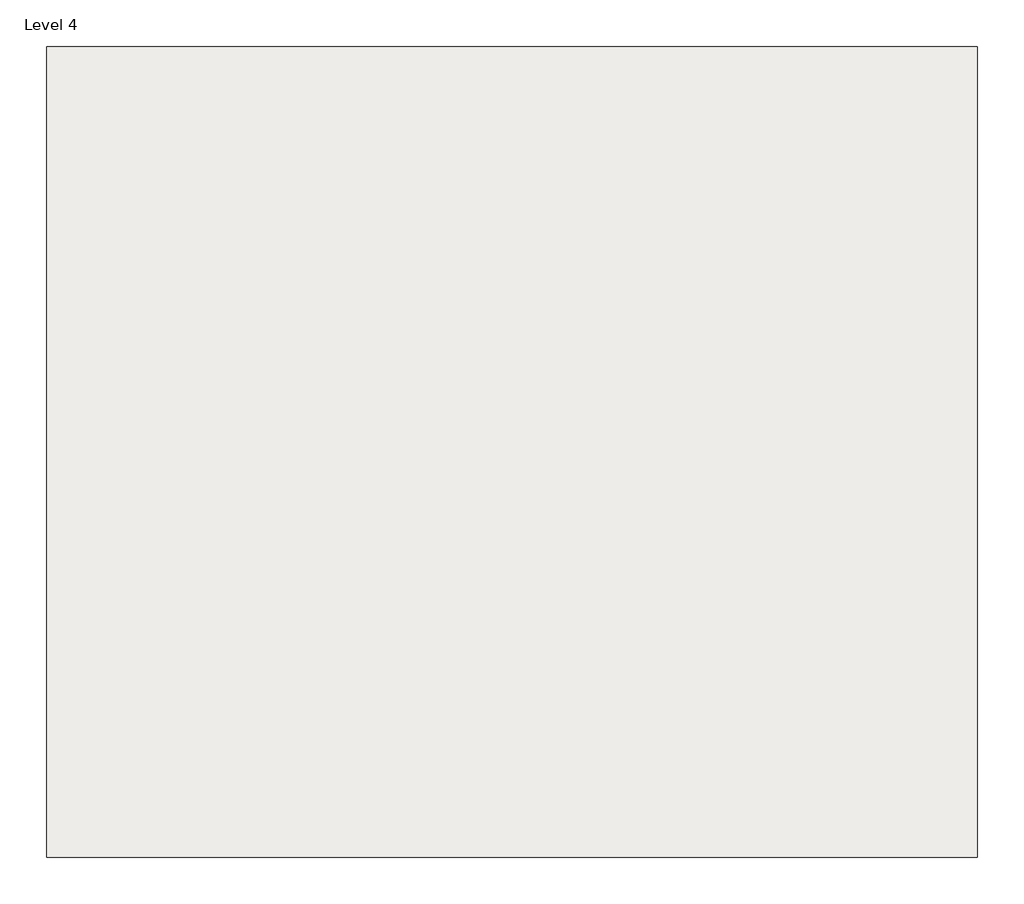
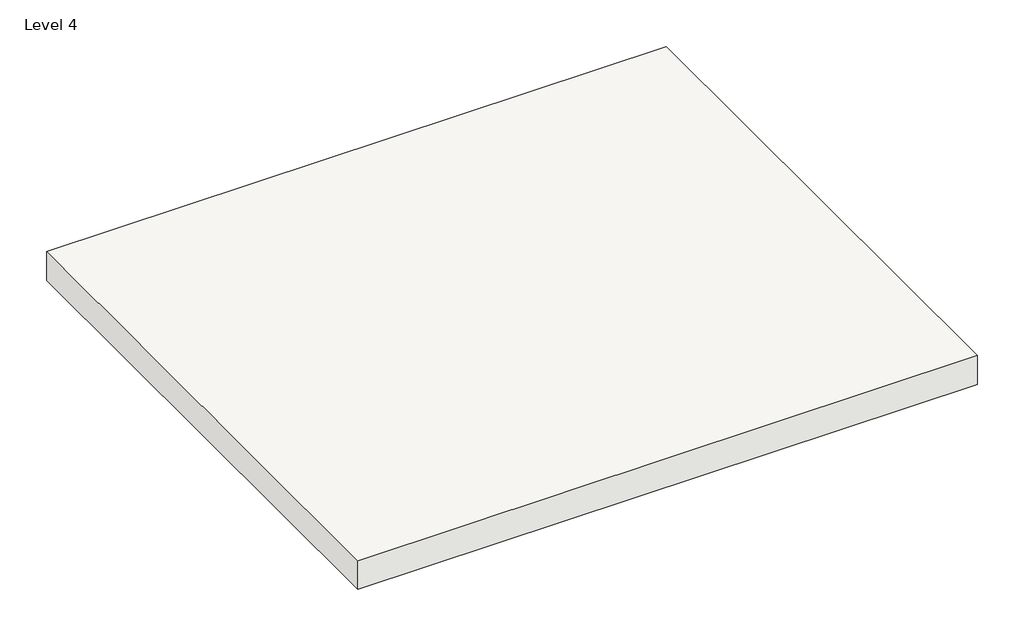
# One storey: 1 roof.
"""IFC4 building model written with IfcOpenShell, lengths in millimetres."""

from ifc_helpers import new_model, si_unit, frame, origin, place, context, project, spatial, polyline, outline, extrude, element, save

model = new_model("IFC4")

# Units and contexts
model_context = context("Model", 3, world=origin())
ifc_project = project(units=[si_unit("LENGTHUNIT", "METRE", prefix="MILLI")], contexts=[model_context])

# Site, building, storey
site = spatial("IfcSite", under=ifc_project)
building = spatial("IfcBuilding", under=site)
storey = spatial("IfcBuildingStorey", under=building, Name="Level 4", Elevation=10972.8)

# Roof
placement = place(None, origin())
element("IfcRoof", 1, ObjectType="Generic - 12\"", at=placement, inside=storey, context=model_context, shape_type="SweptSolid", body=[
    extrude(outline(polyline([(-6240.9183714, 5364.6900371), (-49.6683714, 5364.6900371), (-49.6683714, -26.4599629), (-6240.9183714, -26.4599629), (-6240.9183714, 5364.6900371)])), frame((0.0, 0.0, 9448.8), z_axis=(0.0, 0.0, 1.0), x_axis=(1.0, 0.0, 0.0)), (0.0, 0.0, 1.0), 304.8),
])

save(model, "model.ifc")

# Revit data of these elements
# Type "Generic - 12\""
#   Assembly Code = "B1020"
#   Layers, outside or top first: 1' - 0" no material (function 1)
# Element 1 (IfcRoof, "Generic - 12\"")
#   built-in parameter 1001705 = 32 (stored number, unit not read)
#   built-in parameter 1001701 = -5 (stored number, unit not read)
#   built-in parameter 1001710 = 33615
#   Phase Created = New Construction
#   Materials on its faces: "Default Roof"
# Materials
#   "Default Roof": colour RGB 88 101 114, transparency 0
